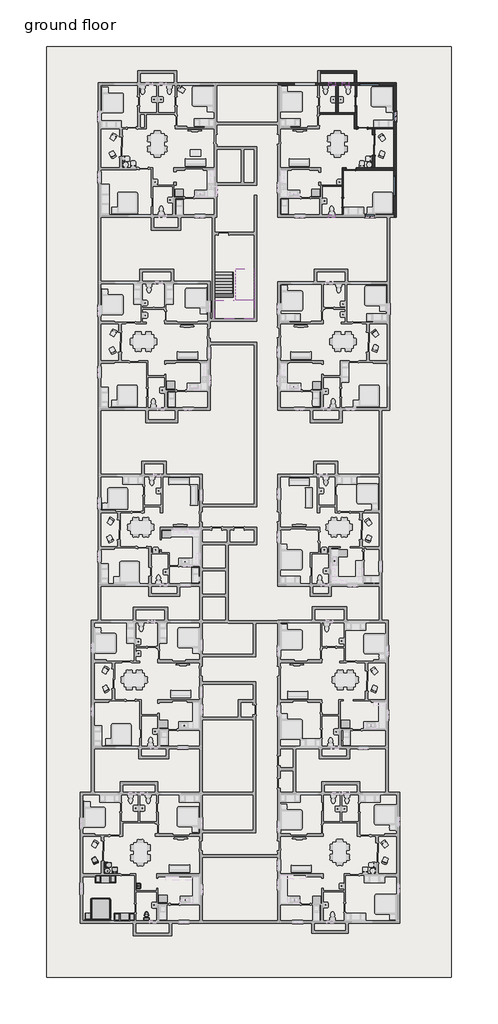
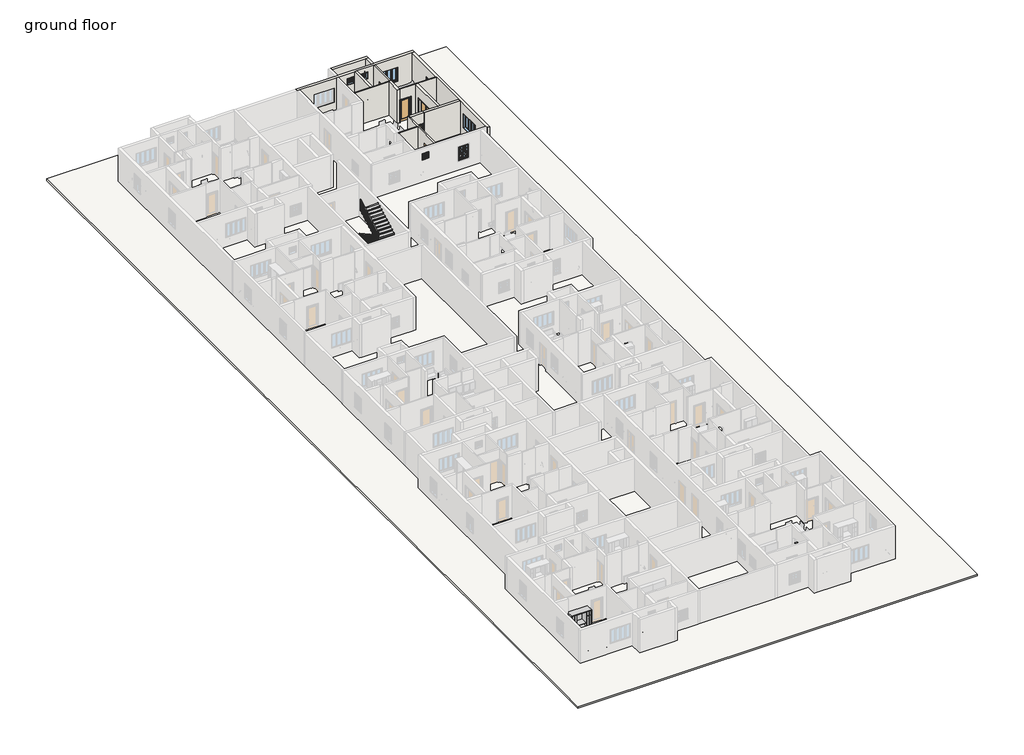
# One storey, part 10 of 16: 15 walls, 7 furniture elements, 7 windows, 5 doors, 2 flow terminals, 2 slabs, 2 stair flights, 1 railing.
"""IFC4 building model written with IfcOpenShell, lengths in millimetres."""

from ifc_helpers import new_model, si_unit, frame, origin, place, context, project, spatial, polyline, outline, extrude, faceted_brep, transform, mapped, element, save
from components import door_d4d75d1e, door_3c6ab76a, door_9c4ddfbd, door_bb092f7c, door_d141acb4, flow_terminal_8d9ea526, toilet_domestic_3d_toilet_domestic_3d_ba6479b0, toilet_domestic_3d_toilet_domestic_3d_30431060, bed_design_8999_bed_design_8999_9c973422, bed_design_8999_bed_design_8999_e911dec7, furniture_88072bd9, furniture_eb3a3c23, furniture_9d41381f, non_monolithic_landing_4cda9577, stair_flight_ae9a2714, stair_flight_a36623a9, window_5487fb6d, window_f2d8fef0, window_45970670

model = new_model("IFC4")

# Units and contexts
model_context = context("Model", 3, world=origin())
ifc_project = project(units=[si_unit("LENGTHUNIT", "METRE", prefix="MILLI")], contexts=[model_context])

# Site, building, storey
site = spatial("IfcSite", under=ifc_project)
building = spatial("IfcBuilding", under=site)
storey = spatial("IfcBuildingStorey", under=building, Name="ground floor", Elevation=609.6)

# Doors
placement = place(None, origin())
door_shape = door_d4d75d1e(model_context)
element("IfcDoor", 1, ObjectType="Door-Double-Sliding : 72\" x 84\"", at=placement, inside=storey, context=model_context, shape_type="MappedRepresentation", body=[
    mapped(door_shape, transform((67904.1483329, 44966.9310851, 609.6), x_axis=(0.0, -1.0, 0.0), y_axis=(1.0, 0.0, 0.0), z_axis=(0.0, 0.0, 1.0))),
])
door_2_shape = door_3c6ab76a(model_context)
element("IfcDoor", 2, ObjectType="Door-Interior-Single-1_Panel-Wood : 36\" x 84\"", at=placement, inside=storey, context=model_context, shape_type="MappedRepresentation", body=[
    mapped(door_2_shape, transform((66996.0226571, 46494.1060851, 609.6), x_axis=(1.0, 0.0, 0.0), y_axis=(0.0, 1.0, 0.0), z_axis=(0.0, 0.0, 1.0))),
])
door_3_shape = door_9c4ddfbd(model_context)
element("IfcDoor", 3, ObjectType="Door-Interior-Single-1_Panel-Wood : 36\" x 84\"", at=placement, inside=storey, context=model_context, shape_type="MappedRepresentation", body=[
    mapped(door_3_shape, transform((65990.3757323, 42800.9047667, 609.6), x_axis=(-1.0, 0.0, 0.0), y_axis=(0.0, -1.0, 0.0), z_axis=(0.0, 0.0, 1.0))),
])
door_4_shape = door_bb092f7c(model_context)
element("IfcDoor", 4, ObjectType="Single-Flush : 32\" x 84\"", at=placement, inside=storey, context=model_context, shape_type="MappedRepresentation", body=[
    mapped(door_4_shape, transform((66424.5226571, 48940.3773256, 609.6), x_axis=(0.0, -1.0, 0.0), y_axis=(1.0, 0.0, 0.0), z_axis=(0.0, 0.0, 1.0))),
])
door_5_shape = door_d141acb4(model_context)
element("IfcDoor", 5, ObjectType="Single-Flush : 32\" x 84\"", at=placement, inside=storey, context=model_context, shape_type="MappedRepresentation", body=[
    mapped(door_5_shape, transform((65228.3757323, 39767.0809867, 609.6), x_axis=(0.0, 1.0, 0.0), y_axis=(-1.0, 0.0, 0.0), z_axis=(0.0, 0.0, 1.0))),
])

# Flow terminals
flow_terminal_shape = flow_terminal_8d9ea526(model_context)
element("IfcFlowTerminal", 6, ObjectType="Sink Vanity-Square : 20\" x 18\"", at=placement, inside=storey, context=model_context, shape_type="MappedRepresentation", body=[
    mapped(flow_terminal_shape, transform((46725.7157736, -21997.351898, 609.6), x_axis=(0.0, 1.0, 0.0), y_axis=(-1.0, 0.0, 0.0), z_axis=(0.0, 0.0, 1.0))),
])
toilet_domestic_3d_toilet_domestic_3d_shape = toilet_domestic_3d_toilet_domestic_3d_ba6479b0(model_context)
toilet_domestic_3d_toilet_domestic_3d_2_shape = toilet_domestic_3d_toilet_domestic_3d_30431060(model_context)
element("IfcFlowTerminal", 7, ObjectType="Toilet-Domestic-3D : Toilet-Domestic-3D", at=placement, inside=storey, context=model_context, shape_type="MappedRepresentation", body=[
    mapped(toilet_domestic_3d_toilet_domestic_3d_shape, transform((47504.076243, -24626.1405635, 609.6), x_axis=(-1.0, 0.0, 0.0), y_axis=(0.0, -1.0, 0.0), z_axis=(0.0, 0.0, 1.0))),
    mapped(toilet_domestic_3d_toilet_domestic_3d_2_shape, transform((47504.076243, -24626.1405635, 609.6), x_axis=(-1.0, 0.0, 0.0), y_axis=(0.0, -1.0, 0.0), z_axis=(0.0, 0.0, 1.0))),
])

# Furniture
bed_design_8999_bed_design_8999_shape = bed_design_8999_bed_design_8999_9c973422(model_context)
bed_design_8999_bed_design_8999_2_shape = bed_design_8999_bed_design_8999_e911dec7(model_context)
element("IfcFurniture", 8, ObjectType="BED_DESIGN_8999 : BED_DESIGN_8999", at=placement, inside=storey, context=model_context, shape_type="MappedRepresentation", body=[
    mapped(bed_design_8999_bed_design_8999_shape, transform((43167.026243, -23088.8358289, 609.6), x_axis=(-1.0, 0.0, 0.0), y_axis=(0.0, -1.0, 0.0), z_axis=(0.0, 0.0, 1.0))),
    mapped(bed_design_8999_bed_design_8999_2_shape, transform((43167.026243, -23088.8358289, 609.6), x_axis=(-1.0, 0.0, 0.0), y_axis=(0.0, -1.0, 0.0), z_axis=(0.0, 0.0, 1.0))),
])
furniture_shape = furniture_88072bd9(model_context)
element("IfcFurniture", 9, ObjectType="Entertainment Center : 72\" x 72\" x 24\"", at=placement, inside=storey, context=model_context, shape_type="MappedRepresentation", body=[
    mapped(furniture_shape, transform((45516.526243, -25222.4365909, 609.6), x_axis=(-1.0, 0.0, 0.0), y_axis=(0.0, -1.0, 0.0), z_axis=(0.0, 0.0, 1.0))),
])
element("IfcFurniture", 10, ObjectType="Entertainment Center : 72\" x 72\" x 24\"", at=placement, inside=storey, context=model_context, shape_type="MappedRepresentation", body=[
    mapped(furniture_shape, transform((43795.676243, -20917.1365909, 609.6), x_axis=(1.0, 0.0, 0.0), y_axis=(0.0, 1.0, 0.0), z_axis=(0.0, 0.0, 1.0))),
])
furniture_2_shape = furniture_eb3a3c23(model_context)
element("IfcFurniture", 11, ObjectType="Seating-Auditorium : 18\" x 24\" x 30\"", at=placement, inside=storey, context=model_context, shape_type="MappedRepresentation", body=[
    mapped(furniture_2_shape, transform((43812.8672418, -19923.2088345, 609.6), x_axis=(0.0, -1.0, 0.0), y_axis=(1.0, 0.0, 0.0), z_axis=(0.0, 0.0, 1.0))),
])
element("IfcFurniture", 12, ObjectType="Seating-Auditorium : 18\" x 24\" x 30\"", at=placement, inside=storey, context=model_context, shape_type="MappedRepresentation", body=[
    mapped(furniture_2_shape, transform((44477.0147828, -20772.8323698, 609.6), x_axis=(1.0, 0.0, 0.0), y_axis=(0.0, 1.0, 0.0), z_axis=(0.0, 0.0, 1.0))),
])
element("IfcFurniture", 13, ObjectType="Seating-Auditorium : 18\" x 24\" x 30\"", at=placement, inside=storey, context=model_context, shape_type="MappedRepresentation", body=[
    mapped(furniture_2_shape, transform((42784.2789856, -19946.659121, 609.6), x_axis=(0.8974056171641766, 0.4412064803265965, 0.0), y_axis=(-0.4412064803265965, 0.8974056171641766, 0.0), z_axis=(0.0, 0.0, 1.0))),
])
furniture_3_shape = furniture_9d41381f(model_context)
element("IfcFurniture", 14, ObjectType="Table-Trio End : 20\" Diameter", at=placement, inside=storey, context=model_context, shape_type="MappedRepresentation", body=[
    mapped(furniture_3_shape, transform((43966.8524682, -20618.2562257, 609.6), x_axis=(1.0, 0.0, 0.0), y_axis=(0.0, 1.0, 0.0), z_axis=(0.0, 0.0, 1.0))),
])

# Railing
element("IfcRailing", 15, ObjectType="Handrail - Rectangular", at=placement, inside=storey, context=model_context, shape_type="SolidModel", body=[
    faceted_brep([(55336.7072437, 33466.7590238, 1676.4), (55336.7072437, 33466.7590238, 1618.5343477), (55285.9072437, 33466.7590238, 1618.5343477), (55285.9072437, 33466.7590238, 1676.4), (55336.7072437, 31028.3590238, 3006.4363636), (55336.7072437, 30977.5590238, 2976.2798022), (55285.9072437, 30977.5590238, 2976.2798022), (55285.9072437, 31028.3590238, 3006.4363636), (55336.7072437, 31028.3590238, 3048.0), (55336.7072437, 30977.5590238, 2997.2), (55285.9072437, 30977.5590238, 2997.2), (55285.9072437, 31028.3590238, 3048.0), (55336.7072437, 30952.1590238, 3048.0), (55336.7072437, 30952.1590238, 2997.2), (55285.9072437, 30901.3590238, 2997.2), (55285.9072437, 30901.3590238, 3048.0), (55412.9072437, 30952.1590238, 3048.0), (55412.9072437, 30952.1590238, 2997.2), (55412.9072437, 30901.3590238, 2997.2), (55412.9072437, 30901.3590238, 3048.0), (55470.3312819, 30952.1590238, 3048.0), (55521.1312819, 30952.1590238, 2997.2), (55521.1312819, 30901.3590238, 2997.2), (55470.3312819, 30901.3590238, 3048.0), (55470.3312819, 30952.1590238, 3241.9636364), (55521.1312819, 30952.1590238, 3191.1636364), (55521.1312819, 30901.3590238, 3191.1636364), (55470.3312819, 30901.3590238, 3241.9636364), (55546.5312819, 30952.1590238, 3241.9636364), (55546.5312819, 30952.1590238, 3191.1636364), (55597.3312819, 30901.3590238, 3191.1636364), (55597.3312819, 30901.3590238, 3241.9636364), (55546.5312819, 31028.3590238, 3241.9636364), (55546.5312819, 31041.3127197, 3191.1636364), (55597.3312819, 31041.3127197, 3191.1636364), (55597.3312819, 31028.3590238, 3241.9636364), (55546.5312819, 33746.1590238, 4724.4), (55597.3312819, 33746.1590238, 4724.4), (55597.3312819, 33746.1590238, 4666.5343477), (55546.5312819, 33746.1590238, 4666.5343477)], [[[0, 1, 2, 3]], [[1, 0, 4, 5]], [[2, 1, 5, 6]], [[3, 2, 6, 7]], [[0, 3, 7, 4]], [[5, 4, 8, 9]], [[6, 5, 9, 10]], [[7, 6, 10, 11]], [[4, 7, 11, 8]], [[9, 8, 12, 13]], [[10, 9, 13, 14]], [[11, 10, 14, 15]], [[8, 11, 15, 12]], [[13, 12, 16, 17]], [[14, 13, 17, 18]], [[15, 14, 18, 19]], [[12, 15, 19, 16]], [[17, 16, 20, 21]], [[18, 17, 21, 22]], [[19, 18, 22, 23]], [[16, 19, 23, 20]], [[21, 20, 24, 25]], [[22, 21, 25, 26]], [[23, 22, 26, 27]], [[20, 23, 27, 24]], [[25, 24, 28, 29]], [[26, 25, 29, 30]], [[27, 26, 30, 31]], [[24, 27, 31, 28]], [[29, 28, 32, 33]], [[30, 29, 33, 34]], [[31, 30, 34, 35]], [[28, 31, 35, 32]], [[36, 37, 38, 39]], [[33, 32, 36, 39]], [[34, 33, 39, 38]], [[35, 34, 38, 37]], [[32, 35, 37, 36]]]),
    extrude(outline(polyline([(33679.4840238, 4630.1661659), (33679.4840238, 3657.6), (33660.4340238, 3657.6), (33660.4340238, 4619.7752568), (33679.4840238, 4630.1661659)])), frame((55562.4062819, 0.0, 0.0), z_axis=(1.0, 0.0, 0.0), x_axis=(0.0, 1.0, 0.0)), (0.0, 0.0, 1.0), 19.05),
    extrude(outline(polyline([(33577.8840238, 4574.747984), (33577.8840238, 3657.6), (33558.8340238, 3657.6), (33558.8340238, 4564.3570749), (33577.8840238, 4574.747984)])), frame((55562.4062819, 0.0, 0.0), z_axis=(1.0, 0.0, 0.0), x_axis=(0.0, 1.0, 0.0)), (0.0, 0.0, 1.0), 19.05),
    extrude(outline(polyline([(33476.2840238, 4519.3298022), (33476.2840238, 3657.6), (33457.2340238, 3657.6), (33457.2340238, 4508.9388931), (33476.2840238, 4519.3298022)])), frame((55562.4062819, 0.0, 0.0), z_axis=(1.0, 0.0, 0.0), x_axis=(0.0, 1.0, 0.0)), (0.0, 0.0, 1.0), 19.05),
    extrude(outline(polyline([(33374.6840238, 4463.9116204), (33374.6840238, 3505.2), (33355.6340238, 3505.2), (33355.6340238, 4453.5207113), (33374.6840238, 4463.9116204)])), frame((55562.4062819, 0.0, 0.0), z_axis=(1.0, 0.0, 0.0), x_axis=(0.0, 1.0, 0.0)), (0.0, 0.0, 1.0), 19.05),
    extrude(outline(polyline([(33273.0840238, 4408.4934386), (33273.0840238, 3505.2), (33254.0340238, 3505.2), (33254.0340238, 4398.1025295), (33273.0840238, 4408.4934386)])), frame((55562.4062819, 0.0, 0.0), z_axis=(1.0, 0.0, 0.0), x_axis=(0.0, 1.0, 0.0)), (0.0, 0.0, 1.0), 19.05),
    extrude(outline(polyline([(33171.4840238, 4353.0752568), (33171.4840238, 3352.8), (33152.4340238, 3352.8), (33152.4340238, 4342.6843477), (33171.4840238, 4353.0752568)])), frame((55562.4062819, 0.0, 0.0), z_axis=(1.0, 0.0, 0.0), x_axis=(0.0, 1.0, 0.0)), (0.0, 0.0, 1.0), 19.05),
    extrude(outline(polyline([(33069.8840238, 4297.6570749), (33069.8840238, 3352.8), (33050.8340238, 3352.8), (33050.8340238, 4287.2661659), (33069.8840238, 4297.6570749)])), frame((55562.4062819, 0.0, 0.0), z_axis=(1.0, 0.0, 0.0), x_axis=(0.0, 1.0, 0.0)), (0.0, 0.0, 1.0), 19.05),
    extrude(outline(polyline([(32968.2840238, 4242.2388931), (32968.2840238, 3352.8), (32949.2340238, 3352.8), (32949.2340238, 4231.847984), (32968.2840238, 4242.2388931)])), frame((55562.4062819, 0.0, 0.0), z_axis=(1.0, 0.0, 0.0), x_axis=(0.0, 1.0, 0.0)), (0.0, 0.0, 1.0), 19.05),
    extrude(outline(polyline([(32866.6840238, 4186.8207113), (32866.6840238, 3200.4), (32847.6340238, 3200.4), (32847.6340238, 4176.4298022), (32866.6840238, 4186.8207113)])), frame((55562.4062819, 0.0, 0.0), z_axis=(1.0, 0.0, 0.0), x_axis=(0.0, 1.0, 0.0)), (0.0, 0.0, 1.0), 19.05),
    extrude(outline(polyline([(32765.0840238, 4131.4025295), (32765.0840238, 3200.4), (32746.0340238, 3200.4), (32746.0340238, 4121.0116204), (32765.0840238, 4131.4025295)])), frame((55562.4062819, 0.0, 0.0), z_axis=(1.0, 0.0, 0.0), x_axis=(0.0, 1.0, 0.0)), (0.0, 0.0, 1.0), 19.05),
    extrude(outline(polyline([(32663.4840238, 4075.9843477), (32663.4840238, 3200.4), (32644.4340238, 3200.4), (32644.4340238, 4065.5934386), (32663.4840238, 4075.9843477)])), frame((55562.4062819, 0.0, 0.0), z_axis=(1.0, 0.0, 0.0), x_axis=(0.0, 1.0, 0.0)), (0.0, 0.0, 1.0), 19.05),
    extrude(outline(polyline([(32561.8840238, 4020.5661659), (32561.8840238, 3048.0), (32542.8340238, 3048.0), (32542.8340238, 4010.1752568), (32561.8840238, 4020.5661659)])), frame((55562.4062819, 0.0, 0.0), z_axis=(1.0, 0.0, 0.0), x_axis=(0.0, 1.0, 0.0)), (0.0, 0.0, 1.0), 19.05),
    extrude(outline(polyline([(32460.2840238, 3965.147984), (32460.2840238, 3048.0), (32441.2340238, 3048.0), (32441.2340238, 3954.7570749), (32460.2840238, 3965.147984)])), frame((55562.4062819, 0.0, 0.0), z_axis=(1.0, 0.0, 0.0), x_axis=(0.0, 1.0, 0.0)), (0.0, 0.0, 1.0), 19.05),
    extrude(outline(polyline([(32358.6840238, 3909.7298022), (32358.6840238, 3048.0), (32339.6340238, 3048.0), (32339.6340238, 3899.3388931), (32358.6840238, 3909.7298022)])), frame((55562.4062819, 0.0, 0.0), z_axis=(1.0, 0.0, 0.0), x_axis=(0.0, 1.0, 0.0)), (0.0, 0.0, 1.0), 19.05),
    extrude(outline(polyline([(32257.0840238, 3854.3116204), (32257.0840238, 2895.6), (32238.0340238, 2895.6), (32238.0340238, 3843.9207113), (32257.0840238, 3854.3116204)])), frame((55562.4062819, 0.0, 0.0), z_axis=(1.0, 0.0, 0.0), x_axis=(0.0, 1.0, 0.0)), (0.0, 0.0, 1.0), 19.05),
    extrude(outline(polyline([(32155.4840238, 3798.8934386), (32155.4840238, 2895.6), (32136.4340238, 2895.6), (32136.4340238, 3788.5025295), (32155.4840238, 3798.8934386)])), frame((55562.4062819, 0.0, 0.0), z_axis=(1.0, 0.0, 0.0), x_axis=(0.0, 1.0, 0.0)), (0.0, 0.0, 1.0), 19.05),
    extrude(outline(polyline([(32053.8840238, 3743.4752568), (32053.8840238, 2743.2), (32034.8340238, 2743.2), (32034.8340238, 3733.0843477), (32053.8840238, 3743.4752568)])), frame((55562.4062819, 0.0, 0.0), z_axis=(1.0, 0.0, 0.0), x_axis=(0.0, 1.0, 0.0)), (0.0, 0.0, 1.0), 19.05),
    extrude(outline(polyline([(31952.2840238, 3688.0570749), (31952.2840238, 2743.2), (31933.2340238, 2743.2), (31933.2340238, 3677.6661659), (31952.2840238, 3688.0570749)])), frame((55562.4062819, 0.0, 0.0), z_axis=(1.0, 0.0, 0.0), x_axis=(0.0, 1.0, 0.0)), (0.0, 0.0, 1.0), 19.05),
    extrude(outline(polyline([(31850.6840238, 3632.6388931), (31850.6840238, 2743.2), (31831.6340238, 2743.2), (31831.6340238, 3622.247984), (31850.6840238, 3632.6388931)])), frame((55562.4062819, 0.0, 0.0), z_axis=(1.0, 0.0, 0.0), x_axis=(0.0, 1.0, 0.0)), (0.0, 0.0, 1.0), 19.05),
    extrude(outline(polyline([(31749.0840238, 3577.2207113), (31749.0840238, 2590.8), (31730.0340238, 2590.8), (31730.0340238, 3566.8298022), (31749.0840238, 3577.2207113)])), frame((55562.4062819, 0.0, 0.0), z_axis=(1.0, 0.0, 0.0), x_axis=(0.0, 1.0, 0.0)), (0.0, 0.0, 1.0), 19.05),
    extrude(outline(polyline([(31647.4840238, 3521.8025295), (31647.4840238, 2590.8), (31628.4340238, 2590.8), (31628.4340238, 3511.4116204), (31647.4840238, 3521.8025295)])), frame((55562.4062819, 0.0, 0.0), z_axis=(1.0, 0.0, 0.0), x_axis=(0.0, 1.0, 0.0)), (0.0, 0.0, 1.0), 19.05),
    extrude(outline(polyline([(31545.8840238, 3466.3843477), (31545.8840238, 2590.8), (31526.8340238, 2590.8), (31526.8340238, 3455.9934386), (31545.8840238, 3466.3843477)])), frame((55562.4062819, 0.0, 0.0), z_axis=(1.0, 0.0, 0.0), x_axis=(0.0, 1.0, 0.0)), (0.0, 0.0, 1.0), 19.05),
    extrude(outline(polyline([(31444.2840238, 3410.9661659), (31444.2840238, 2438.4), (31425.2340238, 2438.4), (31425.2340238, 3400.5752568), (31444.2840238, 3410.9661659)])), frame((55562.4062819, 0.0, 0.0), z_axis=(1.0, 0.0, 0.0), x_axis=(0.0, 1.0, 0.0)), (0.0, 0.0, 1.0), 19.05),
    extrude(outline(polyline([(31342.6840238, 3355.547984), (31342.6840238, 2438.4), (31323.6340238, 2438.4), (31323.6340238, 3345.1570749), (31342.6840238, 3355.547984)])), frame((55562.4062819, 0.0, 0.0), z_axis=(1.0, 0.0, 0.0), x_axis=(0.0, 1.0, 0.0)), (0.0, 0.0, 1.0), 19.05),
    extrude(outline(polyline([(31241.0840238, 3300.1298022), (31241.0840238, 2438.4), (31222.0340238, 2438.4), (31222.0340238, 3289.7388931), (31241.0840238, 3300.1298022)])), frame((55562.4062819, 0.0, 0.0), z_axis=(1.0, 0.0, 0.0), x_axis=(0.0, 1.0, 0.0)), (0.0, 0.0, 1.0), 19.05),
    extrude(outline(polyline([(31139.4840238, 3244.7116204), (31139.4840238, 2286.0), (31120.4340238, 2286.0), (31120.4340238, 3234.3207113), (31139.4840238, 3244.7116204)])), frame((55562.4062819, 0.0, 0.0), z_axis=(1.0, 0.0, 0.0), x_axis=(0.0, 1.0, 0.0)), (0.0, 0.0, 1.0), 19.05),
    extrude(outline(polyline([(31037.8840238, 3189.2934386), (31037.8840238, 2286.0), (31018.8340238, 2286.0), (31018.8340238, 3178.9025295), (31037.8840238, 3189.2934386)])), frame((55562.4062819, 0.0, 0.0), z_axis=(1.0, 0.0, 0.0), x_axis=(0.0, 1.0, 0.0)), (0.0, 0.0, 1.0), 19.05),
    extrude(outline(polyline([(55504.9822437, 30936.2840238), (55524.0322437, 30936.2840238), (55524.0322437, 30917.2340238), (55504.9822437, 30917.2340238), (55504.9822437, 30936.2840238)])), frame((0.0, 0.0, 2133.6), z_axis=(0.0, 0.0, 1.0), x_axis=(1.0, 0.0, 0.0)), (0.0, 0.0, 1.0), 1057.5636364),
    extrude(outline(polyline([(55403.3822437, 30936.2840238), (55422.4322437, 30936.2840238), (55422.4322437, 30917.2340238), (55403.3822437, 30917.2340238), (55403.3822437, 30936.2840238)])), frame((0.0, 0.0, 2133.6), z_axis=(0.0, 0.0, 1.0), x_axis=(1.0, 0.0, 0.0)), (0.0, 0.0, 1.0), 863.6),
    extrude(outline(polyline([(31037.8840238, 2943.3752568), (31037.8840238, 1981.2), (31018.8340238, 1981.2), (31018.8340238, 2953.7661659), (31037.8840238, 2943.3752568)])), frame((55301.7822437, 0.0, 0.0), z_axis=(1.0, 0.0, 0.0), x_axis=(0.0, 1.0, 0.0)), (0.0, 0.0, 1.0), 19.05),
    extrude(outline(polyline([(31139.4840238, 2887.9570749), (31139.4840238, 1981.2), (31120.4340238, 1981.2), (31120.4340238, 2898.347984), (31139.4840238, 2887.9570749)])), frame((55301.7822437, 0.0, 0.0), z_axis=(1.0, 0.0, 0.0), x_axis=(0.0, 1.0, 0.0)), (0.0, 0.0, 1.0), 19.05),
    extrude(outline(polyline([(31241.0840238, 2832.5388931), (31241.0840238, 1981.2), (31222.0340238, 1981.2), (31222.0340238, 2842.9298022), (31241.0840238, 2832.5388931)])), frame((55301.7822437, 0.0, 0.0), z_axis=(1.0, 0.0, 0.0), x_axis=(0.0, 1.0, 0.0)), (0.0, 0.0, 1.0), 19.05),
    extrude(outline(polyline([(31342.6840238, 2777.1207113), (31342.6840238, 1828.8), (31323.6340238, 1828.8), (31323.6340238, 2787.5116204), (31342.6840238, 2777.1207113)])), frame((55301.7822437, 0.0, 0.0), z_axis=(1.0, 0.0, 0.0), x_axis=(0.0, 1.0, 0.0)), (0.0, 0.0, 1.0), 19.05),
    extrude(outline(polyline([(31444.2840238, 2721.7025295), (31444.2840238, 1828.8), (31425.2340238, 1828.8), (31425.2340238, 2732.0934386), (31444.2840238, 2721.7025295)])), frame((55301.7822437, 0.0, 0.0), z_axis=(1.0, 0.0, 0.0), x_axis=(0.0, 1.0, 0.0)), (0.0, 0.0, 1.0), 19.05),
    extrude(outline(polyline([(31545.8840238, 2666.2843477), (31545.8840238, 1676.4), (31526.8340238, 1676.4), (31526.8340238, 2676.6752568), (31545.8840238, 2666.2843477)])), frame((55301.7822437, 0.0, 0.0), z_axis=(1.0, 0.0, 0.0), x_axis=(0.0, 1.0, 0.0)), (0.0, 0.0, 1.0), 19.05),
    extrude(outline(polyline([(31647.4840238, 2610.8661659), (31647.4840238, 1676.4), (31628.4340238, 1676.4), (31628.4340238, 2621.2570749), (31647.4840238, 2610.8661659)])), frame((55301.7822437, 0.0, 0.0), z_axis=(1.0, 0.0, 0.0), x_axis=(0.0, 1.0, 0.0)), (0.0, 0.0, 1.0), 19.05),
    extrude(outline(polyline([(31749.0840238, 2555.447984), (31749.0840238, 1676.4), (31730.0340238, 1676.4), (31730.0340238, 2565.8388931), (31749.0840238, 2555.447984)])), frame((55301.7822437, 0.0, 0.0), z_axis=(1.0, 0.0, 0.0), x_axis=(0.0, 1.0, 0.0)), (0.0, 0.0, 1.0), 19.05),
    extrude(outline(polyline([(31850.6840238, 2500.0298022), (31850.6840238, 1524.0), (31831.6340238, 1524.0), (31831.6340238, 2510.4207113), (31850.6840238, 2500.0298022)])), frame((55301.7822437, 0.0, 0.0), z_axis=(1.0, 0.0, 0.0), x_axis=(0.0, 1.0, 0.0)), (0.0, 0.0, 1.0), 19.05),
    extrude(outline(polyline([(31952.2840238, 2444.6116204), (31952.2840238, 1524.0), (31933.2340238, 1524.0), (31933.2340238, 2455.0025295), (31952.2840238, 2444.6116204)])), frame((55301.7822437, 0.0, 0.0), z_axis=(1.0, 0.0, 0.0), x_axis=(0.0, 1.0, 0.0)), (0.0, 0.0, 1.0), 19.05),
    extrude(outline(polyline([(32053.8840238, 2389.1934386), (32053.8840238, 1524.0), (32034.8340238, 1524.0), (32034.8340238, 2399.5843477), (32053.8840238, 2389.1934386)])), frame((55301.7822437, 0.0, 0.0), z_axis=(1.0, 0.0, 0.0), x_axis=(0.0, 1.0, 0.0)), (0.0, 0.0, 1.0), 19.05),
    extrude(outline(polyline([(32155.4840238, 2333.7752568), (32155.4840238, 1371.6), (32136.4340238, 1371.6), (32136.4340238, 2344.1661659), (32155.4840238, 2333.7752568)])), frame((55301.7822437, 0.0, 0.0), z_axis=(1.0, 0.0, 0.0), x_axis=(0.0, 1.0, 0.0)), (0.0, 0.0, 1.0), 19.05),
    extrude(outline(polyline([(32257.0840238, 2278.3570749), (32257.0840238, 1371.6), (32238.0340238, 1371.6), (32238.0340238, 2288.747984), (32257.0840238, 2278.3570749)])), frame((55301.7822437, 0.0, 0.0), z_axis=(1.0, 0.0, 0.0), x_axis=(0.0, 1.0, 0.0)), (0.0, 0.0, 1.0), 19.05),
    extrude(outline(polyline([(32358.6840238, 2222.9388931), (32358.6840238, 1371.6), (32339.6340238, 1371.6), (32339.6340238, 2233.3298022), (32358.6840238, 2222.9388931)])), frame((55301.7822437, 0.0, 0.0), z_axis=(1.0, 0.0, 0.0), x_axis=(0.0, 1.0, 0.0)), (0.0, 0.0, 1.0), 19.05),
    extrude(outline(polyline([(32460.2840238, 2167.5207113), (32460.2840238, 1219.2), (32441.2340238, 1219.2), (32441.2340238, 2177.9116204), (32460.2840238, 2167.5207113)])), frame((55301.7822437, 0.0, 0.0), z_axis=(1.0, 0.0, 0.0), x_axis=(0.0, 1.0, 0.0)), (0.0, 0.0, 1.0), 19.05),
    extrude(outline(polyline([(32561.8840238, 2112.1025295), (32561.8840238, 1219.2), (32542.8340238, 1219.2), (32542.8340238, 2122.4934386), (32561.8840238, 2112.1025295)])), frame((55301.7822437, 0.0, 0.0), z_axis=(1.0, 0.0, 0.0), x_axis=(0.0, 1.0, 0.0)), (0.0, 0.0, 1.0), 19.05),
    extrude(outline(polyline([(32663.4840238, 2056.6843477), (32663.4840238, 1066.8), (32644.4340238, 1066.8), (32644.4340238, 2067.0752568), (32663.4840238, 2056.6843477)])), frame((55301.7822437, 0.0, 0.0), z_axis=(1.0, 0.0, 0.0), x_axis=(0.0, 1.0, 0.0)), (0.0, 0.0, 1.0), 19.05),
    extrude(outline(polyline([(32765.0840238, 2001.2661659), (32765.0840238, 1066.8), (32746.0340238, 1066.8), (32746.0340238, 2011.6570749), (32765.0840238, 2001.2661659)])), frame((55301.7822437, 0.0, 0.0), z_axis=(1.0, 0.0, 0.0), x_axis=(0.0, 1.0, 0.0)), (0.0, 0.0, 1.0), 19.05),
    extrude(outline(polyline([(32866.6840238, 1945.847984), (32866.6840238, 1066.8), (32847.6340238, 1066.8), (32847.6340238, 1956.2388931), (32866.6840238, 1945.847984)])), frame((55301.7822437, 0.0, 0.0), z_axis=(1.0, 0.0, 0.0), x_axis=(0.0, 1.0, 0.0)), (0.0, 0.0, 1.0), 19.05),
    extrude(outline(polyline([(32968.2840238, 1890.4298022), (32968.2840238, 914.4), (32949.2340238, 914.4), (32949.2340238, 1900.8207113), (32968.2840238, 1890.4298022)])), frame((55301.7822437, 0.0, 0.0), z_axis=(1.0, 0.0, 0.0), x_axis=(0.0, 1.0, 0.0)), (0.0, 0.0, 1.0), 19.05),
    extrude(outline(polyline([(33069.8840238, 1835.0116204), (33069.8840238, 914.4), (33050.8340238, 914.4), (33050.8340238, 1845.4025295), (33069.8840238, 1835.0116204)])), frame((55301.7822437, 0.0, 0.0), z_axis=(1.0, 0.0, 0.0), x_axis=(0.0, 1.0, 0.0)), (0.0, 0.0, 1.0), 19.05),
    extrude(outline(polyline([(33171.4840238, 1779.5934386), (33171.4840238, 914.4), (33152.4340238, 914.4), (33152.4340238, 1789.9843477), (33171.4840238, 1779.5934386)])), frame((55301.7822437, 0.0, 0.0), z_axis=(1.0, 0.0, 0.0), x_axis=(0.0, 1.0, 0.0)), (0.0, 0.0, 1.0), 19.05),
    extrude(outline(polyline([(33273.0840238, 1724.1752568), (33273.0840238, 762.0), (33254.0340238, 762.0), (33254.0340238, 1734.5661659), (33273.0840238, 1724.1752568)])), frame((55301.7822437, 0.0, 0.0), z_axis=(1.0, 0.0, 0.0), x_axis=(0.0, 1.0, 0.0)), (0.0, 0.0, 1.0), 19.05),
    extrude(outline(polyline([(33374.6840238, 1668.7570749), (33374.6840238, 762.0), (33355.6340238, 762.0), (33355.6340238, 1679.147984), (33374.6840238, 1668.7570749)])), frame((55301.7822437, 0.0, 0.0), z_axis=(1.0, 0.0, 0.0), x_axis=(0.0, 1.0, 0.0)), (0.0, 0.0, 1.0), 19.05),
    extrude(outline(polyline([(55562.4062819, 30936.2840238), (55581.4562819, 30936.2840238), (55581.4562819, 30917.2340238), (55562.4062819, 30917.2340238), (55562.4062819, 30936.2840238)])), frame((0.0, 0.0, 2133.6), z_axis=(0.0, 0.0, 1.0), x_axis=(1.0, 0.0, 0.0)), (0.0, 0.0, 1.0), 1057.5636364),
    extrude(outline(polyline([(55320.8322437, 30936.2840238), (55320.8322437, 30917.2340238), (55301.7822437, 30917.2340238), (55301.7822437, 30936.2840238), (55320.8322437, 30936.2840238)])), frame((0.0, 0.0, 2133.6), z_axis=(0.0, 0.0, 1.0), x_axis=(1.0, 0.0, 0.0)), (0.0, 0.0, 1.0), 863.6),
    extrude(outline(polyline([(33746.1590238, 4666.5343477), (33746.1590238, 3657.6), (33727.1090238, 3657.6), (33727.1090238, 4656.1434386), (33746.1590238, 4666.5343477)])), frame((55562.4062819, 0.0, 0.0), z_axis=(1.0, 0.0, 0.0), x_axis=(0.0, 1.0, 0.0)), (0.0, 0.0, 1.0), 19.05),
    extrude(outline(polyline([(33466.7590238, 1618.5343477), (33466.7590238, 762.0), (33447.7090238, 762.0), (33447.7090238, 1628.9252568), (33466.7590238, 1618.5343477)])), frame((55301.7822437, 0.0, 0.0), z_axis=(1.0, 0.0, 0.0), x_axis=(0.0, 1.0, 0.0)), (0.0, 0.0, 1.0), 19.05),
])

# Slabs
element("IfcSlab", 16, ObjectType="Generic - 6\"", at=placement, inside=storey, context=model_context, shape_type="SweptSolid", body=[
    extrude(outline(polyline([(75046.96445, 53870.667236), (75046.96445, -30254.132764), (38470.96445, -30254.132764), (38470.96445, 53870.667236), (75046.96445, 53870.667236)])), frame((0.0, 0.0, 304.8), z_axis=(0.0, 0.0, 1.0), x_axis=(1.0, 0.0, 0.0)), (0.0, 0.0, 1.0), 152.4),
])
non_monolithic_landing_shape = non_monolithic_landing_4cda9577(model_context)
element("IfcSlab", 17, ObjectType="Non-Monolithic Landing", at=placement, inside=storey, context=model_context, shape_type="MappedRepresentation", body=[
    mapped(non_monolithic_landing_shape, transform((0.0, 0.0, 0.0), x_axis=(1.0, 0.0, 0.0), y_axis=(0.0, 1.0, 0.0), z_axis=(0.0, 0.0, 1.0))),
])

# Stair flights
stair_flight_shape = stair_flight_ae9a2714(model_context)
element("IfcStairFlight", 18, ObjectType="2\" Tread 1\" Nosing 1/4\" Riser", at=placement, inside=storey, context=model_context, shape_type="MappedRepresentation", body=[
    mapped(stair_flight_shape, transform((0.0, 0.0, 0.0), x_axis=(1.0, 0.0, 0.0), y_axis=(0.0, 1.0, 0.0), z_axis=(0.0, 0.0, 1.0))),
])
stair_flight_2_shape = stair_flight_a36623a9(model_context)
element("IfcStairFlight", 19, ObjectType="2\" Tread 1\" Nosing 1/4\" Riser", at=placement, inside=storey, context=model_context, shape_type="MappedRepresentation", body=[
    mapped(stair_flight_2_shape, transform((0.0, 0.0, 0.0), x_axis=(1.0, 0.0, 0.0), y_axis=(0.0, 1.0, 0.0), z_axis=(0.0, 0.0, 1.0))),
])

# Walls
element("IfcWall", 20, ObjectType="Generic - 4.5\"", at=placement, inside=storey, context=model_context, shape_type="Brep", body=[
    faceted_brep([(65171.2257323, 42905.6797667, 609.6), (65171.2257323, 41357.9395295, 609.6), (65171.2257323, 41243.6395295, 609.6), (65171.2257323, 40173.4809867, 609.6), (65171.2257323, 40173.4809867, 2743.2), (65171.2257323, 39360.6809867, 2743.2), (65171.2257323, 39360.6809867, 609.6), (65171.2257323, 38662.1809867, 609.6), (65171.2257323, 38662.1809867, 3810.0), (65171.2257323, 41243.6395295, 3810.0), (65171.2257323, 41357.9395295, 3810.0), (65171.2257323, 42905.6797667, 3810.0), (65285.5257323, 40173.4809867, 2743.2), (65285.5257323, 40173.4809867, 609.6), (65285.5257323, 42702.4797667, 609.6), (65285.5257323, 42905.6797667, 609.6), (65285.5257323, 42905.6797667, 3810.0), (65285.5257323, 42702.4797667, 3810.0), (65285.5257323, 38662.1809867, 3810.0), (65285.5257323, 38662.1809867, 609.6), (65285.5257323, 39360.6809867, 609.6), (65285.5257323, 39360.6809867, 2743.2)], [[[0, 1, 2, 3, 4, 5, 6, 7, 8, 9, 10, 11]], [[12, 13, 14, 15, 16, 17, 18, 19, 20, 21]], [[20, 19, 7, 6]], [[15, 14, 13, 3, 2, 1, 0]], [[11, 10, 9, 8, 18, 17, 16]], [[8, 7, 19, 18]], [[0, 11, 16, 15]], [[4, 3, 13, 12]], [[5, 4, 12, 21]], [[6, 5, 21, 20]]]),
])
element("IfcWall", 21, ObjectType="Generic - 4.5\"", at=placement, inside=storey, context=model_context, shape_type="SweptSolid", body=[
    extrude(outline(polyline([(65171.2257323, 41243.6395295), (63382.3476633, 41243.6395295), (63382.3476633, 41357.9395295), (65171.2257323, 41357.9395295), (65171.2257323, 41243.6395295)])), frame((0.0, 0.0, 609.6), z_axis=(0.0, 0.0, 1.0), x_axis=(1.0, 0.0, 0.0)), (0.0, 0.0, 1.0), 3200.4),
])
element("IfcWall", 22, ObjectType="Generic - 4.5\"", at=placement, inside=storey, context=model_context, shape_type="Brep", body=[
    faceted_brep([(66500.7226571, 46548.0810851, 3810.0), (69856.4363207, 46548.0810851, 3810.0), (69856.4363207, 46548.0810851, 609.6), (67478.6226571, 46548.0810851, 609.6), (67478.6226571, 46548.0810851, 2768.6), (66513.4226571, 46548.0810851, 2768.6), (66513.4226571, 46548.0810851, 609.6), (66500.7226571, 46548.0810851, 609.6), (69856.4363207, 46433.7810851, 3810.0), (68145.4483329, 46433.7810851, 3810.0), (67916.8483329, 46433.7810851, 3810.0), (66500.7226571, 46433.7810851, 3810.0), (66500.7226571, 46433.7810851, 609.6), (66513.4226571, 46433.7810851, 609.6), (66513.4226571, 46433.7810851, 2768.6), (67478.6226571, 46433.7810851, 2768.6), (67478.6226571, 46433.7810851, 609.6), (67916.8483329, 46433.7810851, 609.6), (68145.4483329, 46433.7810851, 609.6), (69856.4363207, 46433.7810851, 609.6)], [[[0, 1, 2, 3, 4, 5, 6, 7]], [[8, 9, 10, 11, 12, 13, 14, 15, 16, 17, 18, 19]], [[2, 19, 18, 17, 16, 3]], [[12, 7, 6, 13]], [[1, 0, 11, 10, 9, 8]], [[0, 7, 12, 11]], [[2, 1, 8, 19]], [[15, 4, 3, 16]], [[4, 15, 14, 5]], [[5, 14, 13, 6]]]),
])
element("IfcWall", 23, ObjectType="Generic - 4.5\"", at=placement, inside=storey, context=model_context, shape_type="Brep", body=[
    faceted_brep([(63127.2711425, 47759.2773256, 609.6), (66272.1226571, 47759.2773256, 609.6), (66272.1226571, 47759.2773256, 3810.0), (63127.2711425, 47759.2773256, 3810.0), (63127.2711425, 47873.5773256, 609.6), (63127.2711425, 47873.5773256, 3810.0), (64618.7871882, 47873.5773256, 3810.0), (64821.9871882, 47873.5773256, 3810.0), (66272.1226571, 47873.5773256, 3810.0), (66272.1226571, 47873.5773256, 609.6), (64821.9871882, 47873.5773256, 609.6), (64618.7871882, 47873.5773256, 609.6)], [[[0, 1, 2, 3]], [[4, 5, 6, 7, 8, 9, 10, 11]], [[1, 0, 4, 11, 10, 9]], [[3, 2, 8, 7, 6, 5]], [[2, 1, 9, 8]], [[0, 3, 5, 4]]]),
])
element("IfcWall", 24, ObjectType="Generic - 6\"", at=placement, inside=storey, context=model_context, shape_type="SweptSolid", body=[
    extrude(outline(polyline([(48533.9773256, 2743.2), (48533.9773256, 609.6), (47873.5773256, 609.6), (47873.5773256, 3810.0), (50354.4390836, 3810.0), (50354.4390836, 609.6), (49346.7773256, 609.6), (49346.7773256, 2743.2), (48533.9773256, 2743.2)])), frame((66348.3226571, 0.0, 0.0), z_axis=(1.0, 0.0, 0.0), x_axis=(0.0, 1.0, 0.0)), (0.0, 0.0, 1.0), 152.4),
])
element("IfcWall", 25, ObjectType="Generic - 8\"", at=placement, inside=storey, context=model_context, shape_type="SweptSolid", body=[
    extrude(outline(polyline([(64618.7871882, 47873.5773256), (64618.7871882, 50354.4390836), (64821.9871882, 50354.4390836), (64821.9871882, 47873.5773256), (64618.7871882, 47873.5773256)])), frame((0.0, 0.0, 609.6), z_axis=(0.0, 0.0, 1.0), x_axis=(1.0, 0.0, 0.0)), (0.0, 0.0, 1.0), 3200.4),
])
element("IfcWall", 26, ObjectType="Generic - 8\"", at=placement, inside=storey, context=model_context, shape_type="SweptSolid", body=[
    extrude(outline(polyline([(66553.6297889, 42905.6797667), (69856.4363207, 42905.6797667), (69856.4363207, 42702.4797667), (66553.6297889, 42702.4797667), (66553.6297889, 42905.6797667)])), frame((0.0, 0.0, 609.6), z_axis=(0.0, 0.0, 1.0), x_axis=(1.0, 0.0, 0.0)), (0.0, 0.0, 1.0), 3200.4),
])
element("IfcWall", 27, ObjectType="Generic - 8\"", at=placement, inside=storey, context=model_context, shape_type="SweptSolid", body=[
    extrude(outline(polyline([(3810.0, 69856.4363207), (3810.0, 65285.5257323), (609.6, 65285.5257323), (609.6, 65507.7757323), (2768.6, 65507.7757323), (2768.6, 66472.9757323), (609.6, 66472.9757323), (609.6, 69856.4363207), (3810.0, 69856.4363207)])), frame((0.0, 42702.4797667, 0.0), z_axis=(0.0, 1.0, 0.0), x_axis=(0.0, 0.0, 1.0)), (0.0, 0.0, 1.0), 203.2),
])
element("IfcWall", 28, ObjectType="Generic - 9\"", at=placement, inside=storey, context=model_context, shape_type="Brep", body=[
    faceted_brep([(59356.5312819, 50354.4390836, 609.6), (59585.1312819, 50354.4390836, 609.6), (62974.8711425, 50354.4390836, 609.6), (63127.2711425, 50354.4390836, 609.6), (64618.7871882, 50354.4390836, 609.6), (64821.9871882, 50354.4390836, 609.6), (66348.3226571, 50354.4390836, 609.6), (66500.7226571, 50354.4390836, 609.6), (69856.4363207, 50354.4390836, 609.6), (70085.0363207, 50354.4390836, 609.6), (70085.0363207, 50354.4390836, 3810.0), (69856.4363207, 50354.4390836, 3810.0), (66500.7226571, 50354.4390836, 3810.0), (66348.3226571, 50354.4390836, 3810.0), (64821.9871882, 50354.4390836, 3810.0), (64618.7871882, 50354.4390836, 3810.0), (63127.2711425, 50354.4390836, 3810.0), (62974.8711425, 50354.4390836, 3810.0), (59585.1312819, 50354.4390836, 3810.0), (59356.5312819, 50354.4390836, 3810.0), (62746.2711425, 50354.4390836, 2870.2), (62746.2711425, 50354.4390836, 1524.0), (60917.4711425, 50354.4390836, 1524.0), (60917.4711425, 50354.4390836, 2870.2), (68558.1226571, 50354.4390836, 2870.2), (68558.1226571, 50354.4390836, 1524.0), (66729.3226571, 50354.4390836, 1524.0), (66729.3226571, 50354.4390836, 2870.2), (63958.3871882, 50354.4390836, 3352.8), (64567.9871882, 50354.4390836, 3352.8), (64567.9871882, 50354.4390836, 2743.2), (63958.3871882, 50354.4390836, 2743.2), (65177.5871882, 50354.4390836, 3352.8), (65787.1871882, 50354.4390836, 3352.8), (65787.1871882, 50354.4390836, 2743.2), (65177.5871882, 50354.4390836, 2743.2), (59356.5312819, 50583.0390836, 609.6), (59356.5312819, 50583.0390836, 3810.0), (62967.836417, 50583.0390836, 3810.0), (63196.436417, 50583.0390836, 3810.0), (66272.1226571, 50583.0390836, 3810.0), (66500.7226571, 50583.0390836, 3810.0), (70085.0363207, 50583.0390836, 3810.0), (70085.0363207, 50583.0390836, 609.6), (66500.7226571, 50583.0390836, 609.6), (66272.1226571, 50583.0390836, 609.6), (63196.436417, 50583.0390836, 609.6), (62967.836417, 50583.0390836, 609.6), (62746.2711425, 50583.0390836, 2870.2), (60917.4711425, 50583.0390836, 2870.2), (60917.4711425, 50583.0390836, 1524.0), (62746.2711425, 50583.0390836, 1524.0), (68558.1226571, 50583.0390836, 2870.2), (66729.3226571, 50583.0390836, 2870.2), (66729.3226571, 50583.0390836, 1524.0), (68558.1226571, 50583.0390836, 1524.0), (63958.3871882, 50583.0390836, 3352.8), (63958.3871882, 50583.0390836, 2743.2), (64567.9871882, 50583.0390836, 2743.2), (64567.9871882, 50583.0390836, 3352.8), (65177.5871882, 50583.0390836, 3352.8), (65177.5871882, 50583.0390836, 2743.2), (65787.1871882, 50583.0390836, 2743.2), (65787.1871882, 50583.0390836, 3352.8)], [[[0, 1, 2, 3, 4, 5, 6, 7, 8, 9, 10, 11, 12, 13, 14, 15, 16, 17, 18, 19], [20, 21, 22, 23], [24, 25, 26, 27], [28, 29, 30, 31], [32, 33, 34, 35]], [[36, 37, 38, 39, 40, 41, 42, 43, 44, 45, 46, 47], [48, 49, 50, 51], [52, 53, 54, 55], [56, 57, 58, 59], [60, 61, 62, 63]], [[9, 8, 7, 6, 5, 4, 3, 2, 1, 0, 36, 47, 46, 45, 44, 43]], [[19, 18, 17, 16, 15, 14, 13, 12, 11, 10, 42, 41, 40, 39, 38, 37]], [[10, 9, 43, 42]], [[0, 19, 37, 36]], [[21, 20, 48, 51]], [[22, 21, 51, 50]], [[23, 22, 50, 49]], [[20, 23, 49, 48]], [[25, 24, 52, 55]], [[26, 25, 55, 54]], [[27, 26, 54, 53]], [[24, 27, 53, 52]], [[57, 56, 28, 31]], [[58, 57, 31, 30]], [[59, 58, 30, 29]], [[56, 59, 29, 28]], [[61, 60, 32, 35]], [[62, 61, 35, 34]], [[63, 62, 34, 33]], [[60, 63, 33, 32]]]),
])
element("IfcWall", 29, ObjectType="Generic - 9\"", at=placement, inside=storey, context=model_context, shape_type="Brep", body=[
    faceted_brep([(69856.4363207, 50354.4390836, 609.6), (69856.4363207, 46548.0810851, 609.6), (69856.4363207, 46433.7810851, 609.6), (69856.4363207, 42905.6797667, 609.6), (69856.4363207, 42702.4797667, 609.6), (69856.4363207, 42677.0797667, 609.6), (69856.4363207, 38662.1809867, 609.6), (69856.4363207, 38433.5809867, 609.6), (69856.4363207, 38433.5809867, 3810.0), (69856.4363207, 38662.1809867, 3810.0), (69856.4363207, 42677.0797667, 3810.0), (69856.4363207, 42702.4797667, 3810.0), (69856.4363207, 42905.6797667, 3810.0), (69856.4363207, 46433.7810851, 3810.0), (69856.4363207, 46548.0810851, 3810.0), (69856.4363207, 50354.4390836, 3810.0), (69856.4363207, 40352.9797667, 2870.2), (69856.4363207, 40352.9797667, 1524.0), (69856.4363207, 42181.7797667, 1524.0), (69856.4363207, 42181.7797667, 2870.2), (69856.4363207, 48014.9310851, 2844.8), (69856.4363207, 47100.5310851, 2844.8), (69856.4363207, 47100.5310851, 1524.0), (69856.4363207, 48014.9310851, 1524.0), (70085.0363207, 50354.4390836, 609.6), (70085.0363207, 50354.4390836, 3810.0), (70085.0363207, 38433.5809867, 3810.0), (70085.0363207, 38433.5809867, 609.6), (70085.0363207, 40352.9797667, 2870.2), (70085.0363207, 42181.7797667, 2870.2), (70085.0363207, 42181.7797667, 1524.0), (70085.0363207, 40352.9797667, 1524.0), (70085.0363207, 48014.9310851, 2844.8), (70085.0363207, 48014.9310851, 1524.0), (70085.0363207, 47100.5310851, 1524.0), (70085.0363207, 47100.5310851, 2844.8)], [[[0, 1, 2, 3, 4, 5, 6, 7, 8, 9, 10, 11, 12, 13, 14, 15], [16, 17, 18, 19], [20, 21, 22, 23]], [[24, 25, 26, 27], [28, 29, 30, 31], [32, 33, 34, 35]], [[7, 6, 5, 4, 3, 2, 1, 0, 24, 27]], [[15, 14, 13, 12, 11, 10, 9, 8, 26, 25]], [[0, 15, 25, 24]], [[8, 7, 27, 26]], [[17, 16, 28, 31]], [[18, 17, 31, 30]], [[19, 18, 30, 29]], [[16, 19, 29, 28]], [[33, 32, 20, 23]], [[34, 33, 23, 22]], [[35, 34, 22, 21]], [[32, 35, 21, 20]]]),
])
element("IfcWall", 30, ObjectType="Generic - 9\"", at=placement, inside=storey, context=model_context, shape_type="Brep", body=[
    faceted_brep([(66500.7226571, 46433.7810851, 609.6), (66500.7226571, 46548.0810851, 609.6), (66500.7226571, 47873.5773256, 609.6), (66500.7226571, 47873.5773256, 3810.0), (66500.7226571, 46548.0810851, 3810.0), (66500.7226571, 46433.7810851, 3810.0), (66272.1226571, 46433.7810851, 609.6), (66272.1226571, 46433.7810851, 3810.0), (66272.1226571, 47759.2773256, 3810.0), (66272.1226571, 47873.5773256, 3810.0), (66272.1226571, 47873.5773256, 609.6), (66272.1226571, 47759.2773256, 609.6), (66348.3226571, 47873.5773256, 609.6), (66348.3226571, 47873.5773256, 3810.0)], [[[0, 1, 2, 3, 4, 5]], [[6, 7, 8, 9, 10, 11]], [[2, 1, 0, 6, 11, 10, 12]], [[5, 4, 3, 13, 9, 8, 7]], [[0, 5, 7, 6]], [[3, 2, 12, 10, 9, 13]]]),
])
element("IfcWall", 31, ObjectType="Generic - 9\"", at=placement, inside=storey, context=model_context, shape_type="SweptSolid", body=[
    extrude(outline(polyline([(44052.5310851, 2743.2), (44052.5310851, 609.6), (42905.6797667, 609.6), (42905.6797667, 3810.0), (46433.7810851, 3810.0), (46433.7810851, 609.6), (45881.3310851, 609.6), (45881.3310851, 2743.2), (44052.5310851, 2743.2)])), frame((67916.8483329, 0.0, 0.0), z_axis=(1.0, 0.0, 0.0), x_axis=(0.0, 1.0, 0.0)), (0.0, 0.0, 1.0), 228.6),
])
element("IfcWall", 32, ObjectType="Generic - 9\"", at=placement, inside=storey, context=model_context, shape_type="Brep", body=[
    faceted_brep([(69856.4363207, 42905.6797667, 609.6), (68145.4483329, 42905.6797667, 609.6), (67916.8483329, 42905.6797667, 609.6), (66553.6297889, 42905.6797667, 609.6), (66553.6297889, 42905.6797667, 3810.0), (67916.8483329, 42905.6797667, 3810.0), (68145.4483329, 42905.6797667, 3810.0), (69856.4363207, 42905.6797667, 3810.0), (69856.4363207, 42677.0797667, 609.6), (69856.4363207, 42677.0797667, 3810.0), (66553.6297889, 42677.0797667, 3810.0), (66553.6297889, 42677.0797667, 609.6)], [[[0, 1, 2, 3, 4, 5, 6, 7]], [[8, 9, 10, 11]], [[3, 2, 1, 0, 8, 11]], [[4, 3, 11, 10]], [[7, 6, 5, 4, 10, 9]], [[0, 7, 9, 8]]]),
])
element("IfcWall", 33, ObjectType="Generic - 9\"", at=placement, inside=storey, context=model_context, shape_type="Brep", body=[
    faceted_brep([(63196.436417, 51470.3211687, 609.6), (66272.1226571, 51470.3211687, 609.6), (66500.7226571, 51470.3211687, 609.6), (66500.7226571, 51470.3211687, 3810.0), (66272.1226571, 51470.3211687, 3810.0), (63196.436417, 51470.3211687, 3810.0), (63196.436417, 51698.9211687, 609.6), (63196.436417, 51698.9211687, 3810.0), (66500.7226571, 51698.9211687, 3810.0), (66500.7226571, 51698.9211687, 609.6)], [[[0, 1, 2, 3, 4, 5]], [[6, 7, 8, 9]], [[2, 1, 0, 6, 9]], [[5, 4, 3, 8, 7]], [[0, 5, 7, 6]], [[3, 2, 9, 8]]]),
])
element("IfcWall", 34, ObjectType="Generic - 9\"", at=placement, inside=storey, context=model_context, shape_type="SweptSolid", body=[
    extrude(outline(polyline([(66272.1226571, 50583.0390836), (66272.1226571, 51470.3211687), (66500.7226571, 51470.3211687), (66500.7226571, 50583.0390836), (66272.1226571, 50583.0390836)])), frame((0.0, 0.0, 609.6), z_axis=(0.0, 0.0, 1.0), x_axis=(1.0, 0.0, 0.0)), (0.0, 0.0, 1.0), 3200.4),
])

# Windows
window_shape = window_5487fb6d(model_context)
element("IfcWindow", 35, ObjectType="Window-Casement-Multi-Sash-Horizontal : 72\" x 53\"", at=placement, inside=storey, context=model_context, shape_type="MappedRepresentation", body=[
    mapped(window_shape, transform((67643.7226571, 50468.7390836, 609.6), x_axis=(1.0, 0.0, 0.0), y_axis=(0.0, 1.0, 0.0), z_axis=(0.0, 0.0, 1.0))),
])
element("IfcWindow", 36, ObjectType="Window-Casement-Multi-Sash-Horizontal : 72\" x 53\"", at=placement, inside=storey, context=model_context, shape_type="MappedRepresentation", body=[
    mapped(window_shape, transform((69970.7363207, 41267.3797667, 609.6), x_axis=(0.0, -1.0, 0.0), y_axis=(1.0, 0.0, 0.0), z_axis=(0.0, 0.0, 1.0))),
])
window_2_shape = window_f2d8fef0(model_context)
element("IfcWindow", 37, ObjectType="Window-Louvers : 24\" x 24\"", at=placement, inside=storey, context=model_context, shape_type="MappedRepresentation", body=[
    mapped(window_2_shape, transform((64263.1871882, 50475.0890836, 1828.8), x_axis=(1.0, 0.0, 0.0), y_axis=(0.0, 1.0, 0.0), z_axis=(0.0, 0.0, 1.0))),
])
element("IfcWindow", 38, ObjectType="Window-Louvers : 24\" x 24\"", at=placement, inside=storey, context=model_context, shape_type="MappedRepresentation", body=[
    mapped(window_2_shape, transform((65482.3871882, 50475.0890836, 1828.8), x_axis=(1.0, 0.0, 0.0), y_axis=(0.0, 1.0, 0.0), z_axis=(0.0, 0.0, 1.0))),
])
element("IfcWindow", 39, ObjectType="Window-Louvers : 24\" x 24\"", at=placement, inside=storey, context=model_context, shape_type="MappedRepresentation", body=[
    mapped(window_2_shape, transform((64239.1744479, 38541.5309867, 1828.8), x_axis=(-1.0, 0.0, 0.0), y_axis=(0.0, -1.0, 0.0), z_axis=(0.0, 0.0, 1.0))),
])
window_3_shape = window_45970670(model_context)
element("IfcWindow", 40, ObjectType="Window-Single-Hung-Double : 36\" x 52\"", at=placement, inside=storey, context=model_context, shape_type="MappedRepresentation", body=[
    mapped(window_3_shape, transform((67687.7312819, 38547.8809867, 609.6), x_axis=(-1.0, 0.0, 0.0), y_axis=(0.0, -1.0, 0.0), z_axis=(0.0, 0.0, 1.0))),
])
element("IfcWindow", 41, ObjectType="Window-Single-Hung-Double : 36\" x 52\"", at=placement, inside=storey, context=model_context, shape_type="MappedRepresentation", body=[
    mapped(window_3_shape, transform((69970.7363207, 47557.7310851, 609.6), x_axis=(0.0, -1.0, 0.0), y_axis=(1.0, 0.0, 0.0), z_axis=(0.0, 0.0, 1.0))),
])

save(model, "model.ifc")

# Revit data of these elements
# Type "Door-Double-Sliding : 72\" x 84\""
#   Type Mark = "12"
#   Construction Type Id = "opn-d45"
#   Assembly Code = "C1020"
#   Analytic Construction = "Wood frame, double glass door "
#   Thickness = 0' - 2"
#   Thermal Resistance (R) = 1.8150 (h·ft²·°F)/BTU
#   Heat Transfer Coefficient (U) = 0.5510 BTU/(h·ft²·°F)
#   Height = 7' - 0"
#   Rail Width = 0' - 2"
#   Stiles = 0' - 2"
#   Trim Projection Ext = 0' - 1"
#   Trim Projection Int = 0' - 1"
#   Trim Width = 0' - 3"
#   Width = 6' - 0"
#   Define Thermal Properties by = 1
#   Glazing = Glass
#   Panel Material = Wood - Birch - Solid Stained Light Low Gloss
#   Trim Material = Paint - Sienna
#   Visual Light Transmittance = 0
#   Solar Heat Gain Coefficient = 0
#   Function = (empty or 0)
#   Wall Closure = (empty or 0)
# Type "Door-Interior-Single-1_Panel-Wood : 36\" x 84\""
#   Type Mark = "8"
#   Assembly Code = "C1020300"
#   Analytic Construction = "Wooden"
#   Top Rail = 0' - 4 11/16"
#   Thickness = 0' - 1 3/8"
#   Thermal Resistance (R) = 2.5876 (h·ft²·°F)/BTU
#   Swing Angle [instance default] = 90.00°
#   Stiles = 0' - 4 3/4"
#   Rough Width = 3' - 2"
#   Rough Height = 7' - 1"
#   Height = 7' - 0"
#   Width = 3' - 0"
#   Heat Transfer Coefficient (U) = 0.3865 BTU/(h·ft²·°F)
#   Bottom Rail = 0' - 9 1/8"
#   Trim Material = Cherry
#   Panel Material = Cherry
#   Frame Material = Cherry
#   Door Handle Material = Aluminum
#   Visual Light Transmittance = 0
#   Solar Heat Gain Coefficient = 0
#   Wall Closure = (empty or 0)
#   Function = (empty or 0)
# Type "Single-Flush : 32\" x 84\""
#   Type Mark = "3"
#   Construction Type Id = "MDOOR"
#   Assembly Code = "C1020"
#   Analytic Construction = "Metal"
#   Thickness = 0' - 2"
#   Heat Transfer Coefficient (U) = 0.651978 BTU/(h·ft²·°F)
#   Height = 7' - 0"
#   Trim Projection Ext = 0' - 1"
#   Trim Projection Int = 0' - 1"
#   Trim Width = 0' - 3"
#   Width = 2' - 8"
#   Define Thermal Properties by = 1
#   Define Thermal Properties by = 1
#   Door Material = Door - Panel
#   Frame Material = Door - Frame
#   Visual Light Transmittance = 0
#   Solar Heat Gain Coefficient = 0
#   Function = (empty or 0)
#   Wall Closure = (empty or 0)
# Type "Sink Vanity-Square : 20\" x 18\""
#   Assembly Code = "D2010400"
#   Counter Height = 2' - 7"
#   Depth = 1' - 6"
#   Width = 1' - 8"
#   Basin Material = Porcelain, Linen
#   Faucet Material = Steel, Polished
#   Default Elevation = 0
# Type "Toilet-Domestic-3D : Toilet-Domestic-3D"
#   Assembly Code = "D2010110"
#   Toilet - Bowl/Basin Material = Porcelain, Linen
#   Toilet - Seat Material = Laminate, Linen, Matte
#   Default Elevation = 0
# Type "BED_DESIGN_8999 : BED_DESIGN_8999"
#   Default Elevation = 0
# Type "Entertainment Center : 72\" x 72\" x 24\""
#   Assembly Code = "E2020200"
#   Center Width = 2' - 8"
#   Depth = 2' - 0"
#   Height = 6' - 0"
#   Width = 6' - 0"
#   Material = none
#   Default Elevation = 0
# Type "Seating-Auditorium : 18\" x 24\" x 30\""
#   Assembly Code = "E2020200"
#   Seat Material = Linen, Beige
#   Frame Material = Steel, Paint Finish, Dark Gray, Matte
#   Default Elevation = 0
# Type "Table-Trio End : 20\" Diameter"
#   Assembly Code = "E2020200"
#   Base and Trim Material = Wood - Birch
#   Table Top Material = Laminate - Ivory,Matte
#   Default Elevation = 0
# Type "Handrail - Rectangular"
#   Assembly Code = "C2010400"
#   built-in parameter 1008612 = 0.0416667 (stored number, unit not read)
#   built-in parameter 1008611 = 0.0416667 (stored number, unit not read)
#   built-in parameter 1008609 = 0.333333 (stored number, unit not read)
#   built-in parameter 1008604 = 0.166667 (stored number, unit not read)
#   built-in parameter 1008603 = 0.166667 (stored number, unit not read)
#   Railing Height = 3' - 0"
#   built-in parameter 1008630 = 2
#   built-in parameter 1008610 = 2
#   built-in parameter 1008618 = Baluster - Square : 3/4"
# Type "Generic - 6\""
#   Assembly Code = "B1010"
#   Function = 0
#   Layers, outside or top first: 0' - 6" no material (function 1)
# Type "Generic - 4.5\""
#   Assembly Code = "B2010"
#   Layers, outside or top first: 0' - 4 1/2" no material (function 1)
# Type "Generic - 6\""
#   Assembly Code = "B2010"
#   Layers, outside or top first: 0' - 6" no material (function 1)
# Type "Generic - 8\""
#   Assembly Code = "B2010"
#   Layers, outside or top first: 0' - 8" no material (function 1)
# Type "Generic - 9\""
#   Assembly Code = "B2010"
#   Layers, outside or top first: 0' - 9" no material (function 1)
# Type "Window-Casement-Multi-Sash-Horizontal : 72\" x 53\""
#   Type Mark = "24"
#   Fire Rating = "0.5h"
#   Assembly Code = "B2020100"
#   Analytic Construction = "Double glazing - domestic"
#   Window Inset [instance default] = 0' - 0 5/8"
#   Wall Thickness [instance default] = 0' - 6"
#   Visual Light Transmittance = 0.81
#   Thermal Resistance (R) = 1.8146 (h·ft²·°F)/BTU
#   Solar Heat Gain Coefficient = 0.76
#   Rough Width = 6' - 0 1/2"
#   Rough Height = 4' - 5 1/2"
#   Open Window Width = 1' - 6"
#   Heat Transfer Coefficient (U) = 0.5511 BTU/(h·ft²·°F)
#   Height = 4' - 5"
#   Frame Gap 3 [instance default] = 0' - 1 83/128"
#   Frame Gap 2 [instance default] = 0' - 0 5/8"
#   Frame Gap 1 = 0' - 1 51/128"
#   Default Sill Height = 3' - 0"
#   Width = 6' - 0"
#   Frame Material = Metal - Aluminum
#   Glass Panel Material = Glass
#   Wall Closure = (empty or 0)
# Type "Window-Louvers : 24\" x 24\""
#   Type Mark = "18"
#   Construction Type Id = "GSP4R"
#   Assembly Code = "B20"
#   Analytic Construction = "1/8 in Pilkington single glazing"
#   Visual Light Transmittance = 0.9
#   Thermal Resistance (R) = 1.53941 (h·ft²·°F)/BTU
#   Solar Heat Gain Coefficient = 0.78
#   Max Height = 1' - 11.74264"
#   Height = 2' - 0"
#   Heat Transfer Coefficient (U) = 0.6496 BTU/(h·ft²·°F)
#   Blade Width [instance default] = 1' - 10 1/2"
#   Blade Vertical Thickness = 0' - 0.35355"
#   Blade Thickness = 0' - 0 1/4"
#   Blade Spacing = 0' - 1 1/2"
#   Blade Height = 0' - 1.85355"
#   Blade Depth = 0' - 3"
#   Blade Angle = 45.00°
#   Default Sill Height = 3' - 0"
#   Trim Projection_Exterior = 0' - 0 1/2"
#   Trim Projection_Interior = 0' - 0 1/2"
#   Trim Width_Exterior = 0' - 1 1/2"
#   Trim Width_Interior = 0' - 1 1/2"
#   Width = 2' - 0"
#   Max Blade Count = 12
#   Define Thermal Properties by = 1
#   Blade Count = 12
#   Frame Material = Birch
#   Louver Material = Birch
#   Trim Exterior Material = Birch
#   Trim Interior Material = Birch
#   Wall Closure = (empty or 0)
# Type "Window-Single-Hung-Double : 36\" x 52\""
#   Type Mark = "27"
#   Fire Rating = "0.5h"
#   Construction Type Id = "DG-DR"
#   Assembly Code = "B2020100"
#   Analytic Construction = "Double glazing - domestic"
#   Wall Thickness [instance default] = 0' - 6"
#   Window Inset [instance default] = 0' - 0"
#   Visual Light Transmittance = 0.81
#   Thermal Resistance (R) = 1.8146 (h·ft²·°F)/BTU
#   Solar Heat Gain Coefficient = 0.76
#   Muntin Width = 1' - 0 1/16"
#   Muntin Height = 1' - 10 1/8"
#   Interior Wall Closure [instance default] = 0' - 1 1/2"
#   Rough Width = 3' - 0 1/2"
#   Rough Height = 4' - 4 1/2"
#   Frame Extension [instance default] = 0' - 1 1/4"
#   Exterior Wall Closure [instance default] = 0' - 0 1/2"
#   Extension Jamb [instance default] = 0' - 1 1/2"
#   Heat Transfer Coefficient (U) = 0.5511 BTU/(h·ft²·°F)
#   Height = 4' - 4"
#   Width = 3' - 0"
#   Top Muntin Visibility = yes
#   Indicator Visibility [instance default] = yes
#   Extension Jamb Visibility [instance default] = yes
#   Interior Trim Visibility [instance default] = yes
#   Exterior Trim Visibility [instance default] = yes
#   Define Thermal Properties by = 1
#   Bottom Muntin Visibility = yes
#   Muntin Pattern = Muntin Pattern_2x2 : Muntin Pattern_2x2
#   Interior Trim = Trim-Window-Interior-Flat : Picture Frame
#   Interior Trim Material = Wood - Stained
#   Exterior Trim Material = Clad - White
#   Exterior Trim = Trim-Window-Exterior-Flat : with Sill
#   Glass Panel Material = Glass
#   Exterior Frame Material = Clad - White
#   Interior Frame Material = Wood - Stained
#   Wall Closure = (empty or 0)
# Element 1 (IfcDoor, "Door-Double-Sliding : 72\" x 84\"")
#   Phase Created = New Construction
#   Materials on its faces: "Paint - Sienna", "Wood - Birch - Solid Stained Light Low Gloss", "Glass"
# Elements 2, 3 (IfcDoor, "Door-Interior-Single-1_Panel-Wood : 36\" x 84\"")
#   Swing Angle = 90.00°
#   Phase Created = New Construction
#   Materials on its faces: "Cherry", "Aluminum"
# Elements 4, 5 (IfcDoor, "Single-Flush : 32\" x 84\"")
#   Phase Created = New Construction
#   Materials on its faces: "Door - Frame", "Door - Panel"
# Element 6 (IfcFlowTerminal, "Sink Vanity-Square : 20\" x 18\"")
#   Mark = "47"
#   Phase Created = New Construction
